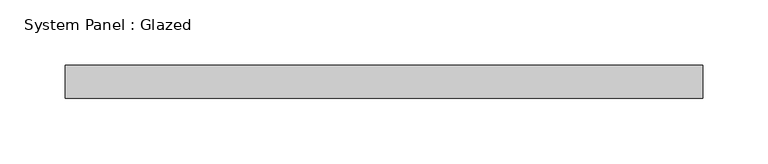
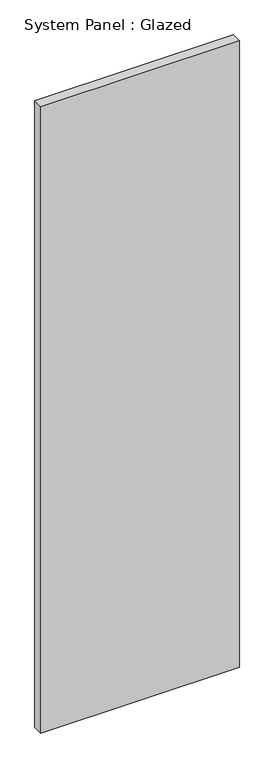
"""IFC4 building model written with IfcOpenShell, lengths in millimetres: plate geometry, System Panel : Glazed."""

from ifc_helpers import new_model, si_unit, origin, origin_with_axes, place, context, project, spatial, polyline, outline, extrude, source, transform, mapped, element, save


def system_panel_glazed_5c179d98(model_context):
    return source(origin(), model_context, "Body", "SweptSolid", [
        extrude(outline(polyline([(244.475, 19.05), (-244.475, 19.05), (-244.475, 44.45), (244.475, 44.45), (244.475, 19.05)])), origin_with_axes(), (0.0, 0.0, 1.0), 1630.093674),
    ])


if __name__ == "__main__":
    model = new_model("IFC4")
    model_context = context("Model", 3, world=origin())
    ifc_project = project(units=[si_unit("LENGTHUNIT", "METRE", prefix="MILLI")], contexts=[model_context])
    site = spatial("IfcSite", under=ifc_project)
    building = spatial("IfcBuilding", under=site)
    placement = place(None, origin())
    system_panel_glazed_shape = system_panel_glazed_5c179d98(model_context)
    element("IfcPlate", 1, ObjectType="System Panel : Glazed", at=placement, inside=building, context=model_context, shape_type="MappedRepresentation", body=[
        mapped(system_panel_glazed_shape, transform((0.0, 0.0, 0.0), x_axis=(1.0, 0.0, 0.0), y_axis=(0.0, 1.0, 0.0), z_axis=(0.0, 0.0, 1.0))),
    ])
    save(model, "model.ifc")

# Revit data of these elements
# Type "System Panel : Glazed"
#   Construction Type Id = "GSP4R"
#   Analytic Construction = "1/8 in Pilkington single glazing"
#   Visual Light Transmittance = 0.9
#   Solar Heat Gain Coefficient = 0.86
#   Heat Transfer Coefficient (U) = 1.18115 BTU/(h·ft²·°F)
#   Define Thermal Properties by = 1
# Element 1 (IfcPlate, "System Panel : Glazed")
#   Materials on its faces: "Glass"
# Materials
#   "Glass": class "Glass", colour RGB 0 128 192, transparency 0.75, Description = "Soda Lime Glass", Cost = 0
